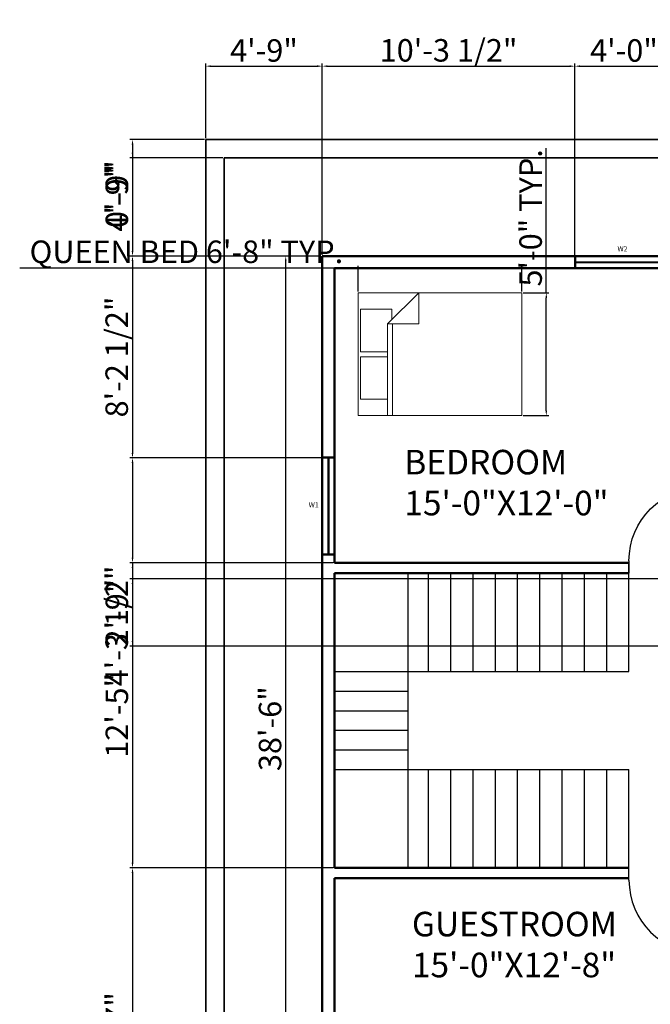
# Model space of a CAD drawing. Units: inches. Extents: x 2299 to 4423, y 1066 to 1805.
# Tile 5 of 7: x 3028 to 3336, y 1315 to 1796. Entities that reach past the tile are written whole.
import ezdxf

# ---------------------------------------------------------------- set-up
doc = ezdxf.new("R2010")
doc.units = ezdxf.units.IN
for name, color, linetype, lineweight in [('A-ANNO-DIMS', 2, 'Continuous', 18), ('A-ANNO-TEXT', 1, 'Continuous', 25), ('A-AREA-IDEN', 1, 'Continuous', 25), ('A-DOOR', 5, 'Continuous', 25), ('A-FLOR-STRS', 6, 'Continuous', 25), ('A-FURN', 8, 'Continuous', 18), ('A-GLAZ', 3, 'Continuous', 25), ('A-WALL', 7, 'Continuous', 50), ('C-PROP', 7, 'Continuous', 35)]:
    doc.layers.add(name, color=color, linetype=linetype, lineweight=lineweight)
doc.styles.get("Standard").update_dxf_attribs({"font": 'arial.ttf'})
doc.dimstyles.new('ISO-25', dxfattribs={"dimtxt": 11, "dimasz": 2.5, "dimexe": 1.25, "dimexo": 0.625, "dimtad": 1, "dimlunit": 4, "dimtxsty": 'Standard', "dimcen": 2.5, "dimadec": 0, "dimazin": 0, "dimtfac": 1, "dimtmove": 0, "dimatfit": 3, "dimfxl": 1, "dimarcsym": 0})

# ---------------------------------------------------------------- blocks, each defined once
blk = doc.blocks.new('*U2')
for p, q in [((0, 0), (0, -5)), ((30, 0), (30, -5))]:
    blk.add_line(p, q)
blk.add_lwpolyline([(0, 0), (0, 30), (1.75, 30), (1.75, 0)], close=True)
blk.add_arc((0, 0), 30, 0, 90)
blk = doc.blocks.new('Bed - Queen')
for p, q in [((0, -80.00003), (0, 0)), ((0, 0), (59.99999, 0)), ((59.99999, 0), (59.99999, -80.00003)), ((7.99999, -1.2), (28.79998, -1.2)), ((7.99999, -14.4), (7.99999, -1.2)), ((28.79998, -1.2), (28.79998, -14.4)), ((31.19999, -1.2), (51.99999, -1.2)), ((31.19999, -14.4), (31.19999, -1.2)), ((51.99999, -1.2), (51.99999, -16.4)), ((0, -14.4), (44.8, -14.4)), ((59.99999, -29.6), (44.8, -14.4)), ((44.8, -14.4), (44.8, -29.6)), ((44.8, -16.8), (0, -16.8)), ((51.99999, -16.4), (46.79936, -16.4)), ((44.8, -29.6), (59.99999, -29.6)), ((59.99999, -80.00003), (0, -80.00003))]:
    blk.add_line(p, q)
blk = doc.blocks.new('*D25')
at = {"layer": 'A-ANNO-DIMS', "color": 0, "lineweight": -2, "transparency": 16777216}
for p, q in [((3175.12, 1680.95), (3156.64, 1680.95)), ((3157.89, 1221.45), (3157.89, 1678.45)), ((3175.12, 1218.95), (3156.64, 1218.95))]:
    blk.add_line(p, q, dxfattribs=at)
at = {"layer": 'A-ANNO-DIMS', "color": 0, "transparency": 16777216}
for points in [[(3157.47, 1678.45), (3158.3, 1678.45), (3157.89, 1680.95)], [(3157.47, 1221.45), (3158.3, 1221.45), (3157.89, 1218.95)]]:
    blk.add_solid(points, dxfattribs=at)
at = {"layer": 'Defpoints', "color": 0, "transparency": 16777216}
for p in [(3157.89, 1680.95), (3175.75, 1680.95), (3175.75, 1218.95)]:
    blk.add_point(p, dxfattribs=at)
at = {"layer": 'A-ANNO-DIMS', "color": 0, "transparency": 16777216, "insert": (3151.64, 1449.95), "char_height": 11, "attachment_point": 5, "rotation": 90}
blk.add_mtext('38\'-6"', dxfattribs=at)
blk = doc.blocks.new('WIN-1200')
for p, q in [((0, 0), (0, 48.07)), ((0, 48.07), (6, 48.07)), ((0, 47.57), (6, 47.57)), ((2.8, 47.57), (2.8, 0.5)), ((3.2, 47.57), (3.2, 0.5)), ((6, 48.07), (6, 0)), ((6, 0.5), (0, 0.5)), ((6, 0), (0, 0))]:
    blk.add_line(p, q)
blk = doc.blocks.new('*D48')
at = {"layer": 'A-ANNO-DIMS', "color": 0, "lineweight": -2, "transparency": 16777216}
for p, q in [((3193.32, 1674.95), (3027.76, 1674.95)), ((3193.32, 1663.57), (3193.32, 1676.2)), ((3270.82, 1674.95), (3195.82, 1674.95)), ((3273.32, 1663.57), (3273.32, 1676.2))]:
    blk.add_line(p, q, dxfattribs=at)
at = {"layer": 'A-ANNO-DIMS', "color": 0, "transparency": 16777216}
for points in [[(3195.82, 1675.36), (3195.82, 1674.53), (3193.32, 1674.95)], [(3270.82, 1675.36), (3270.82, 1674.53), (3273.32, 1674.95)]]:
    blk.add_solid(points, dxfattribs=at)
at = {"layer": 'Defpoints', "color": 0, "transparency": 16777216}
for p in [(3193.32, 1674.95), (3193.32, 1662.95), (3273.32, 1662.95)]:
    blk.add_point(p, dxfattribs=at)
at = {"layer": 'A-ANNO-DIMS', "color": 0, "transparency": 16777216, "insert": (3109.29, 1681.6), "char_height": 11, "attachment_point": 5}
blk.add_mtext('QUEEN BED 6\'-8" TYP.', dxfattribs=at)
blk = doc.blocks.new('*D49')
at = {"layer": 'A-ANNO-DIMS', "color": 0, "lineweight": -2, "transparency": 16777216}
for p, q in [((3285.32, 1662.95), (3285.32, 1733.75)), ((3273.94, 1662.95), (3286.57, 1662.95)), ((3285.32, 1605.45), (3285.32, 1660.45)), ((3273.94, 1602.95), (3286.57, 1602.95))]:
    blk.add_line(p, q, dxfattribs=at)
at = {"layer": 'A-ANNO-DIMS', "color": 0, "transparency": 16777216}
for points in [[(3284.9, 1660.45), (3285.74, 1660.45), (3285.32, 1662.95)], [(3284.9, 1605.45), (3285.74, 1605.45), (3285.32, 1602.95)]]:
    blk.add_solid(points, dxfattribs=at)
at = {"layer": 'Defpoints', "color": 0, "transparency": 16777216}
for p in [(3273.32, 1662.95), (3285.32, 1662.95), (3273.32, 1602.95)]:
    blk.add_point(p, dxfattribs=at)
at = {"layer": 'A-ANNO-DIMS', "color": 0, "transparency": 16777216, "insert": (3279.08, 1699.6), "char_height": 11, "attachment_point": 5, "rotation": 90}
blk.add_mtext('5\'-0" TYP.', dxfattribs=at)
blk = doc.blocks.new('*D61')
at = {"layer": 'A-ANNO-DIMS', "color": 0, "lineweight": -2, "transparency": 16777216}
for p, q in [((3489.68, 1523.12), (3081.7, 1523.12)), ((3082.95, 1520.62), (3082.95, 1492.76)), ((3499.13, 1490.26), (3081.7, 1490.26))]:
    blk.add_line(p, q, dxfattribs=at)
at = {"layer": 'A-ANNO-DIMS', "color": 0, "transparency": 16777216}
for points in [[(3082.53, 1520.62), (3083.37, 1520.62), (3082.95, 1523.12)], [(3082.53, 1492.76), (3083.37, 1492.76), (3082.95, 1490.26)]]:
    blk.add_solid(points, dxfattribs=at)
at = {"layer": 'Defpoints', "color": 0, "transparency": 16777216}
for p in [(3490.3, 1523.12), (3082.95, 1490.26), (3499.76, 1490.26)]:
    blk.add_point(p, dxfattribs=at)
at = {"layer": 'A-ANNO-DIMS', "color": 0, "transparency": 16777216, "insert": (3076.71, 1506.69), "char_height": 11, "attachment_point": 5, "rotation": 90}
blk.add_mtext('2\'-9"', dxfattribs=at)
blk = doc.blocks.new('*D91')
at = {"layer": 'A-ANNO-DIMS', "color": 0, "lineweight": -2, "transparency": 16777216}
for p, q in [((3118.75, 1738.57), (3118.75, 1775)), ((3121.25, 1773.75), (3173.25, 1773.75)), ((3175.75, 1681.57), (3175.75, 1775))]:
    blk.add_line(p, q, dxfattribs=at)
at = {"layer": 'A-ANNO-DIMS', "color": 0, "transparency": 16777216}
for points in [[(3121.25, 1774.16), (3121.25, 1773.33), (3118.75, 1773.75)], [(3173.25, 1774.16), (3173.25, 1773.33), (3175.75, 1773.75)]]:
    blk.add_solid(points, dxfattribs=at)
at = {"layer": 'Defpoints', "color": 0, "transparency": 16777216}
for p in [(3175.75, 1773.75), (3118.75, 1737.95), (3175.75, 1680.95)]:
    blk.add_point(p, dxfattribs=at)
at = {"layer": 'A-ANNO-DIMS', "color": 0, "transparency": 16777216, "insert": (3147.25, 1779.99), "char_height": 11, "attachment_point": 5}
blk.add_mtext('4\'-9"', dxfattribs=at)
blk = doc.blocks.new('*D92')
at = {"layer": 'A-ANNO-DIMS', "color": 0, "lineweight": -2, "transparency": 16777216}
for p, q in [((3175.75, 1681.57), (3175.75, 1775)), ((3178.25, 1773.75), (3296.78, 1773.75)), ((3299.28, 1681.57), (3299.28, 1775))]:
    blk.add_line(p, q, dxfattribs=at)
at = {"layer": 'A-ANNO-DIMS', "color": 0, "transparency": 16777216}
for points in [[(3178.25, 1774.16), (3178.25, 1773.33), (3175.75, 1773.75)], [(3296.78, 1774.16), (3296.78, 1773.33), (3299.28, 1773.75)]]:
    blk.add_solid(points, dxfattribs=at)
at = {"layer": 'Defpoints', "color": 0, "transparency": 16777216}
for p in [(3299.28, 1773.75), (3175.75, 1680.95), (3299.28, 1680.95)]:
    blk.add_point(p, dxfattribs=at)
at = {"layer": 'A-ANNO-DIMS', "color": 0, "transparency": 16777216, "insert": (3237.52, 1780.06), "char_height": 11, "attachment_point": 5}
blk.add_mtext('10\'-3 1/2"', dxfattribs=at)
blk = doc.blocks.new('*D93')
at = {"layer": 'A-ANNO-DIMS', "color": 0, "lineweight": -2, "transparency": 16777216}
for p, q in [((3299.28, 1681.57), (3299.28, 1775)), ((3301.78, 1773.75), (3344.85, 1773.75)), ((3347.35, 1681.57), (3347.35, 1775))]:
    blk.add_line(p, q, dxfattribs=at)
at = {"layer": 'A-ANNO-DIMS', "color": 0, "transparency": 16777216}
for points in [[(3301.78, 1774.16), (3301.78, 1773.33), (3299.28, 1773.75)], [(3344.85, 1774.16), (3344.85, 1773.33), (3347.35, 1773.75)]]:
    blk.add_solid(points, dxfattribs=at)
at = {"layer": 'Defpoints', "color": 0, "transparency": 16777216}
for p in [(3347.35, 1773.75), (3299.28, 1680.95), (3347.35, 1680.95)]:
    blk.add_point(p, dxfattribs=at)
at = {"layer": 'A-ANNO-DIMS', "color": 0, "transparency": 16777216, "insert": (3323.32, 1779.99), "char_height": 11, "attachment_point": 5}
blk.add_mtext('4\'-0"', dxfattribs=at)
blk = doc.blocks.new('*D98')
at = {"layer": 'A-ANNO-DIMS', "color": 0, "lineweight": -2, "transparency": 16777216}
for p, q in [((3118.12, 1737.95), (3081.7, 1737.95)), ((3082.95, 1735.45), (3082.95, 1683.45)), ((3175.12, 1680.95), (3081.7, 1680.95))]:
    blk.add_line(p, q, dxfattribs=at)
at = {"layer": 'A-ANNO-DIMS', "color": 0, "transparency": 16777216}
for points in [[(3082.53, 1735.45), (3083.37, 1735.45), (3082.95, 1737.95)], [(3082.53, 1683.45), (3083.37, 1683.45), (3082.95, 1680.95)]]:
    blk.add_solid(points, dxfattribs=at)
at = {"layer": 'Defpoints', "color": 0, "transparency": 16777216}
for p in [(3118.75, 1737.95), (3082.95, 1680.95), (3175.75, 1680.95)]:
    blk.add_point(p, dxfattribs=at)
at = {"layer": 'A-ANNO-DIMS', "color": 0, "transparency": 16777216, "insert": (3076.71, 1709.45), "char_height": 11, "attachment_point": 5, "rotation": 90}
blk.add_mtext('4\'-9"', dxfattribs=at)
blk = doc.blocks.new('*D99')
at = {"layer": 'A-ANNO-DIMS', "color": 0, "lineweight": -2, "transparency": 16777216}
for p, q in [((3175.12, 1680.95), (3081.7, 1680.95)), ((3082.95, 1678.45), (3082.95, 1584.75)), ((3175.12, 1582.25), (3081.7, 1582.25))]:
    blk.add_line(p, q, dxfattribs=at)
at = {"layer": 'A-ANNO-DIMS', "color": 0, "transparency": 16777216}
for points in [[(3082.53, 1678.45), (3083.37, 1678.45), (3082.95, 1680.95)], [(3082.53, 1584.75), (3083.37, 1584.75), (3082.95, 1582.25)]]:
    blk.add_solid(points, dxfattribs=at)
at = {"layer": 'Defpoints', "color": 0, "transparency": 16777216}
for p in [(3175.75, 1680.95), (3082.95, 1582.25), (3175.75, 1582.25)]:
    blk.add_point(p, dxfattribs=at)
at = {"layer": 'A-ANNO-DIMS', "color": 0, "transparency": 16777216, "insert": (3076.64, 1631.6), "char_height": 11, "attachment_point": 5, "rotation": 90}
blk.add_mtext('8\'-2 1/2"', dxfattribs=at)
blk = doc.blocks.new('*D100')
at = {"layer": 'A-ANNO-DIMS', "color": 0, "lineweight": -2, "transparency": 16777216}
for p, q in [((3175.12, 1582.25), (3081.7, 1582.25)), ((3082.95, 1579.75), (3082.95, 1533.45)), ((3181.12, 1530.95), (3081.7, 1530.95)), ((3082.95, 1530.95), (3082.95, 1471.88))]:
    blk.add_line(p, q, dxfattribs=at)
at = {"layer": 'A-ANNO-DIMS', "color": 0, "transparency": 16777216}
for points in [[(3082.53, 1579.75), (3083.37, 1579.75), (3082.95, 1582.25)], [(3082.53, 1533.45), (3083.37, 1533.45), (3082.95, 1530.95)]]:
    blk.add_solid(points, dxfattribs=at)
at = {"layer": 'Defpoints', "color": 0, "transparency": 16777216}
for p in [(3175.75, 1582.25), (3082.95, 1530.95), (3181.75, 1530.95)]:
    blk.add_point(p, dxfattribs=at)
at = {"layer": 'A-ANNO-DIMS', "color": 0, "transparency": 16777216, "insert": (3076.63, 1500.16), "char_height": 11, "attachment_point": 5, "rotation": 90}
blk.add_mtext('4\'-3 1/2"', dxfattribs=at)
blk = doc.blocks.new('*D101')
at = {"layer": 'A-ANNO-DIMS', "color": 0, "lineweight": -2, "transparency": 16777216}
for p, q in [((3181.12, 1530.95), (3081.7, 1530.95)), ((3082.95, 1528.45), (3082.95, 1384.45)), ((3181.12, 1381.95), (3081.7, 1381.95))]:
    blk.add_line(p, q, dxfattribs=at)
at = {"layer": 'A-ANNO-DIMS', "color": 0, "transparency": 16777216}
for points in [[(3082.53, 1528.45), (3083.37, 1528.45), (3082.95, 1530.95)], [(3082.53, 1384.45), (3083.37, 1384.45), (3082.95, 1381.95)]]:
    blk.add_solid(points, dxfattribs=at)
at = {"layer": 'Defpoints', "color": 0, "transparency": 16777216}
for p in [(3181.75, 1530.95), (3082.95, 1381.95), (3181.75, 1381.95)]:
    blk.add_point(p, dxfattribs=at)
at = {"layer": 'A-ANNO-DIMS', "color": 0, "transparency": 16777216, "insert": (3076.71, 1456.45), "char_height": 11, "attachment_point": 5, "rotation": 90}
blk.add_mtext('12\'-5"', dxfattribs=at)
blk = doc.blocks.new('*D102')
at = {"layer": 'A-ANNO-DIMS', "color": 0, "lineweight": -2, "transparency": 16777216}
for p, q in [((3181.12, 1381.95), (3081.7, 1381.95)), ((3082.95, 1379.45), (3082.95, 1221.45)), ((3175.12, 1218.95), (3081.7, 1218.95))]:
    blk.add_line(p, q, dxfattribs=at)
at = {"layer": 'A-ANNO-DIMS', "color": 0, "transparency": 16777216}
for points in [[(3082.53, 1379.45), (3083.37, 1379.45), (3082.95, 1381.95)], [(3082.53, 1221.45), (3083.37, 1221.45), (3082.95, 1218.95)]]:
    blk.add_solid(points, dxfattribs=at)
at = {"layer": 'Defpoints', "color": 0, "transparency": 16777216}
for p in [(3181.75, 1381.95), (3082.95, 1218.95), (3175.75, 1218.95)]:
    blk.add_point(p, dxfattribs=at)
at = {"layer": 'A-ANNO-DIMS', "color": 0, "transparency": 16777216, "insert": (3076.7, 1300.45), "char_height": 11, "attachment_point": 5, "rotation": 90}
blk.add_mtext('13\'-7"', dxfattribs=at)
blk = doc.blocks.new('*D104')
at = {"layer": 'A-ANNO-DIMS', "color": 0, "lineweight": -2, "transparency": 16777216}
for p, q in [((3118.12, 1737.95), (3081.7, 1737.95)), ((3082.95, 1735.45), (3082.95, 1731.45)), ((3127.12, 1728.95), (3081.7, 1728.95)), ((3082.95, 1728.95), (3082.95, 1695.95))]:
    blk.add_line(p, q, dxfattribs=at)
at = {"layer": 'A-ANNO-DIMS', "color": 0, "transparency": 16777216}
for points in [[(3082.53, 1735.45), (3083.37, 1735.45), (3082.95, 1737.95)], [(3082.53, 1731.45), (3083.37, 1731.45), (3082.95, 1728.95)]]:
    blk.add_solid(points, dxfattribs=at)
at = {"layer": 'Defpoints', "color": 0, "transparency": 16777216}
for p in [(3118.75, 1737.95), (3082.95, 1728.95), (3127.75, 1728.95)]:
    blk.add_point(p, dxfattribs=at)
at = {"layer": 'A-ANNO-DIMS', "color": 0, "transparency": 16777216, "insert": (3076.71, 1711.2), "char_height": 11, "attachment_point": 5, "rotation": 90}
blk.add_mtext('0\'-9"', dxfattribs=at)

msp = doc.modelspace()

# ---------------------------------------------------------------- linework, layer by layer
at = {"layer": 'A-FLOR-STRS'}
for p, q in [((3325.749, 1477.945), (3325.749, 1530.945)), ((3217.749, 1525.945), (3181.749, 1525.945)), ((3181.749, 1525.945), (3181.749, 1381.945)), ((3217.749, 1381.945), (3217.749, 1525.945)), ((3227.749, 1477.945), (3227.749, 1525.945)), ((3238.638, 1477.945), (3238.638, 1525.945)), ((3249.527, 1477.945), (3249.527, 1525.945)), ((3260.416, 1477.945), (3260.416, 1525.945)), ((3271.305, 1477.945), (3271.305, 1525.945)), ((3282.194, 1477.945), (3282.194, 1525.945)), ((3293.082, 1477.945), (3293.082, 1525.945)), ((3303.971, 1477.945), (3303.971, 1525.945)), ((3314.86, 1477.945), (3314.86, 1525.945)), ((3325.749, 1477.945), (3325.749, 1525.945)), ((3181.749, 1477.945), (3325.749, 1477.945)), ((3181.749, 1468.345), (3217.749, 1468.345)), ((3181.749, 1458.745), (3217.749, 1458.745)), ((3181.749, 1449.145), (3217.749, 1449.145)), ((3181.749, 1439.545), (3217.749, 1439.545)), ((3181.749, 1429.945), (3325.749, 1429.945)), ((3181.749, 1429.945), (3325.749, 1429.945)), ((3227.749, 1381.945), (3227.749, 1429.945)), ((3238.638, 1381.945), (3238.638, 1429.945)), ((3249.527, 1381.945), (3249.527, 1429.945)), ((3260.416, 1381.945), (3260.416, 1429.945)), ((3271.305, 1381.945), (3271.305, 1429.945)), ((3282.194, 1381.945), (3282.194, 1429.945)), ((3293.082, 1381.945), (3293.082, 1429.945)), ((3303.971, 1381.945), (3303.971, 1429.945)), ((3314.86, 1381.945), (3314.86, 1429.945)), ((3325.749, 1381.945), (3325.749, 1429.945)), ((3325.749, 1376.945), (3325.749, 1429.945)), ((3181.749, 1381.945), (3217.749, 1381.945))]:
    msp.add_line(p, q, dxfattribs=at)
at = {"layer": 'A-WALL'}
for p, q in [((3175.749, 1218.945), (3175.749, 1680.945)), ((3175.749, 1680.945), (3541.749, 1680.945)), ((3181.749, 1530.945), (3181.749, 1674.945)), ((3181.749, 1674.945), (3325.749, 1674.945)), ((3181.749, 1674.945), (3535.749, 1674.945)), ((3181.749, 1530.945), (3325.749, 1530.945)), ((3181.749, 1381.945), (3181.749, 1525.945)), ((3181.749, 1525.945), (3325.749, 1525.945)), ((3181.749, 1381.945), (3325.749, 1381.945)), ((3181.749, 1224.945), (3181.749, 1376.945)), ((3181.749, 1376.945), (3325.749, 1376.945))]:
    msp.add_line(p, q, dxfattribs=at)
at = {"layer": 'C-PROP'}
for p, q in [((3118.749, 1161.945), (3118.749, 1737.945)), ((3118.749, 1737.945), (3598.749, 1737.945)), ((3127.749, 1170.945), (3127.749, 1728.945)), ((3127.749, 1728.945), (3589.749, 1728.945))]:
    msp.add_line(p, q, dxfattribs=at)

# ---------------------------------------------------------------- block references
at = {"layer": 'A-DOOR', "xscale": -1.199999999999999, "yscale": 1.199999999999999, "zscale": 1.199999999999999}
msp.add_blockref('*U2', (3361.749, 1531.945), dxfattribs=at)
at = {"layer": 'A-DOOR', "xscale": 1.199999999999999, "yscale": 1.199999999999999, "zscale": 1.199999999999999, "rotation": 180}
msp.add_blockref('*U2', (3361.749, 1375.945), dxfattribs=at)
at = {"layer": 'A-FURN', "rotation": 90}
msp.add_blockref('Bed - Queen', (3193.32, 1602.945), dxfattribs=at)
at = {"layer": 'A-GLAZ', "rotation": 90.00000000000188}
msp.add_blockref('WIN-1200', (3347.352, 1674.945), dxfattribs=at)
at = {"layer": 'A-GLAZ'}
msp.add_blockref('WIN-1200', (3175.749, 1534.684), dxfattribs=at)

# ---------------------------------------------------------------- texts
at = {"layer": 'A-ANNO-TEXT', "char_height": 2.5, "attachment_point": 1}
for s, insert in [('W2', (3320.154, 1685.701)), ('W1', (3169.117, 1560.598))]:
    msp.add_mtext(s, dxfattribs=dict(at, insert=insert))
at = {"layer": 'A-AREA-IDEN', "char_height": 12, "attachment_point": 1}
for s, insert in [('BEDROOM\\P15\'-0"X12\'-0"', (3215.895, 1586.224)), ('GUESTROOM\\P15\'-0"X12\'-8"', (3219.595, 1360.434))]:
    msp.add_mtext_dynamic_manual_height_columns(s, width=9.28623, gutter_width=12.5, heights=[0], dxfattribs=dict(at, insert=insert))

# ---------------------------------------------------------------- dimensions: what is measured, and where the dimension line sits
at = {"layer": 'A-ANNO-DIMS'}
for base, p1, p2, picture, middle in [((3299.282, 1773.745), (3175.749, 1680.945), (3299.282, 1680.945), '*D92', (3237.515, 1780.062)), ((3175.749, 1773.745), (3118.749, 1737.945), (3175.749, 1680.945), '*D91', (3147.249, 1779.987)), ((3347.352, 1773.745), (3299.282, 1680.945), (3347.352, 1680.945), '*D93', (3323.317, 1779.987))]:
    dim = msp.add_linear_dim(base=base, p1=p1, p2=p2, dimstyle='ISO-25', override={"dimdec": 1, "dimlfac": 1, "dimrnd": 0, "dimzin": 1, "dimdsep": 46, "dimlunit": 4, "dimfrac": 2}, dxfattribs=at)
    dim.commit()
    dim.dimension.update_dxf_attribs({"geometry": picture, "text_midpoint": middle})
for base, p1, p2, override, picture, middle in [((3082.949, 1680.945), (3118.749, 1737.945), (3175.749, 1680.945), {"dimdec": 1, "dimlfac": 1, "dimrnd": 0, "dimzin": 1, "dimdsep": 46, "dimlunit": 4, "dimfrac": 2}, '*D98', (3076.708, 1709.445)), ((3082.949, 1728.945), (3118.749, 1737.945), (3127.749, 1728.945), {"dimdec": 1, "dimlfac": 1, "dimrnd": 0, "dimzin": 1, "dimdsep": 46, "dimlunit": 4, "dimfrac": 2}, '*D104', (3076.708, 1711.2)), ((3082.949, 1582.255), (3175.749, 1680.945), (3175.749, 1582.255), {"dimdec": 1, "dimlfac": 1, "dimrnd": 0, "dimzin": 1, "dimdsep": 46, "dimlunit": 4, "dimfrac": 2}, '*D99', (3076.637, 1631.6)), ((3157.885, 1680.945), (3175.749, 1218.945), (3175.749, 1680.945), {"dimclrd": 0, "dimclre": 0, "dimclrt": 0}, '*D25', (3151.64, 1449.945)), ((3082.949, 1530.945), (3175.749, 1582.255), (3181.749, 1530.945), {"dimdec": 1, "dimlfac": 1, "dimrnd": 0, "dimzin": 1, "dimdsep": 46, "dimlunit": 4, "dimfrac": 2}, '*D100', (3076.633, 1500.163)), ((3082.949, 1381.945), (3181.749, 1530.945), (3181.749, 1381.945), {"dimdec": 1, "dimlfac": 1, "dimrnd": 0, "dimzin": 1, "dimdsep": 46, "dimlunit": 4, "dimfrac": 2}, '*D101', (3076.708, 1456.445)), ((3082.949, 1490.257), (3490.302, 1523.118), (3499.757, 1490.257), {"dimdec": 1, "dimlfac": 1, "dimrnd": 0, "dimzin": 1, "dimdsep": 46, "dimlunit": 4, "dimfrac": 2}, '*D61', (3076.708, 1506.687)), ((3082.949, 1218.945), (3181.749, 1381.945), (3175.749, 1218.945), {"dimdec": 1, "dimlfac": 1, "dimrnd": 0, "dimzin": 1, "dimdsep": 46, "dimlunit": 4, "dimfrac": 2}, '*D102', (3076.704, 1300.445))]:
    dim = msp.add_linear_dim(base=base, p1=p1, p2=p2, angle=90, dimstyle='ISO-25', override=override, dxfattribs=at)
    dim.commit()
    dim.dimension.update_dxf_attribs({"geometry": picture, "text_midpoint": middle})
for base, p1, p2, angle, text, picture, middle in [((3285.32, 1662.945), (3273.32, 1602.945), (3273.32, 1662.945), 90, '<> TYP.', '*D49', (3279.079, 1699.596)), ((3193.32, 1674.945), (3273.32, 1662.945), (3193.32, 1662.945), 180, 'QUEEN BED <> TYP.', '*D48', (3109.289, 1681.596))]:
    dim = msp.add_linear_dim(base=base, p1=p1, p2=p2, angle=angle, text=text, dimstyle='ISO-25', override={"dimdec": 1, "dimrnd": 0, "dimzin": 1, "dimlunit": 4, "dimfrac": 2}, dxfattribs=at)
    dim.commit()
    dim.dimension.update_dxf_attribs({"geometry": picture, "text_midpoint": middle})

doc.saveas('drawing.dxf')
